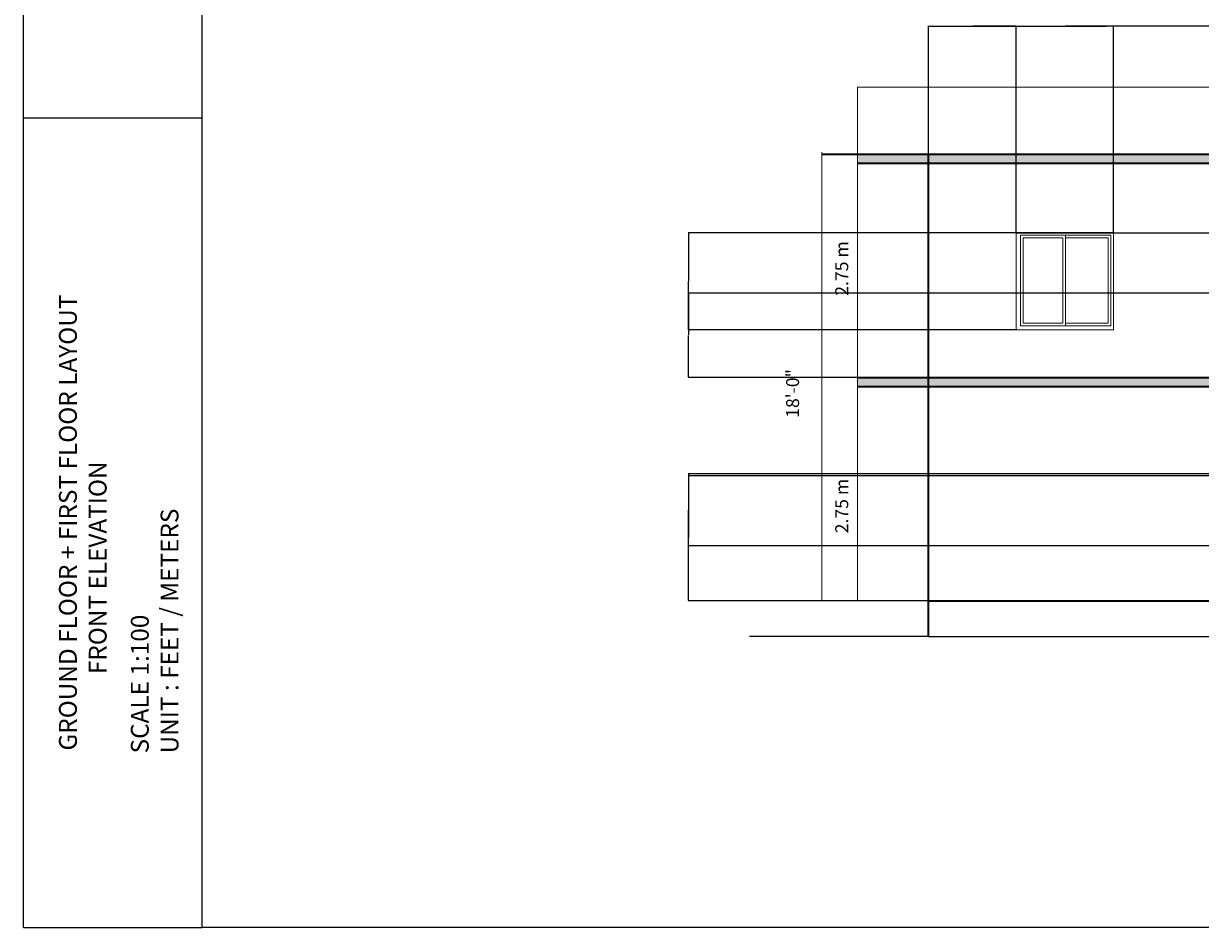
# Model space of a CAD drawing. Units: feet. Extents: x 2813 to 4435, y 1041 to 2557.
# Tile 1 of 6: x 2813 to 3605, y 1041 to 1649. Entities that reach past the tile are written whole.
import ezdxf

# ---------------------------------------------------------------- set-up
doc = ezdxf.new("R2010")
doc.units = ezdxf.units.FT
for name, color, linetype, lineweight in [('A-ANNO-DIMS', 2, 'Continuous', 18), ('A-ANNO-TTLB', 7, 'Continuous', 25), ('A-ELEV', 7, 'Continuous', 35), ('A-ELEV-GRND', 7, 'Continuous', 25), ('A-ELEV-PATT', 252, 'Continuous', 13), ('A-GLAZ', 4, 'Continuous', 18)]:
    doc.layers.add(name, color=color, linetype=linetype, lineweight=lineweight)
doc.styles.get("Standard").update_dxf_attribs({"font": 'arial.ttf'})
doc.dimstyles.get("Standard").update_dxf_attribs({"dimtxt": 0.18, "dimasz": 0.18, "dimexe": 0.18, "dimexo": 0.0625, "dimgap": 0.09, "dimtad": 0, "dimtih": 1, "dimtoh": 1, "dimdec": 4, "dimzin": 0, "dimdsep": 46, "dimtxsty": 'Standard', "dimcen": 0.09, "dimadec": 0, "dimazin": 0, "dimtfac": 1, "dimtdec": 4, "dimtofl": 0, "dimtmove": 0, "dimatfit": 3, "dimfxl": 1, "dimtolj": 1, "dimtzin": 0, "dimarcsym": 0})

# ---------------------------------------------------------------- blocks, each defined once
blk = doc.blocks.new('*U14')
for p, q in [((38.1, 38.1), (38.1, 876.3)), ((38.1, 876.3), (457.2, 876.3)), ((457.2, 38.1), (457.2, 876.3)), ((457.2, 876.3), (876.3, 876.3)), ((876.3, 876.3), (876.3, 38.1)), ((457.2, 38.1), (38.1, 38.1)), ((876.3, 38.1), (457.2, 38.1))]:
    blk.add_line(p, q)
blk.add_lwpolyline([(0, 0), (900, 0), (900, 900), (0, 900)], close=True)
for points in [[(431.8, 850.9), (431.8, 63.5), (63.5, 63.5), (63.5, 850.9), (431.8, 850.9)], [(457.2, 850.9), (850.9, 850.9), (850.9, 63.5), (457.2, 63.5)]]:
    blk.add_lwpolyline(points)
blk = doc.blocks.new('*D35')
at = {"layer": 'A-ANNO-DIMS', "color": 0, "lineweight": -2, "transparency": 16777216}
for p, q in [((3421.71, 1261.18), (3421.71, 1647.39)), ((3421.89, 1647.21), (3541.42, 1647.21)), ((3661.53, 1647.21), (3542, 1647.21)), ((3661.71, 1261.18), (3661.71, 1647.39))]:
    blk.add_line(p, q, dxfattribs=at)
at = {"layer": 'A-ANNO-DIMS', "color": 0, "transparency": 16777216}
for points in [[(3421.89, 1647.24), (3421.89, 1647.18), (3421.71, 1647.21)], [(3661.53, 1647.24), (3661.53, 1647.18), (3661.71, 1647.21)]]:
    blk.add_solid(points, dxfattribs=at)
at = {"layer": 'DEFPOINTS', "color": 0, "transparency": 16777216}
for p in [(3661.71, 1647.21), (3421.71, 1261.11), (3661.71, 1261.11)]:
    blk.add_point(p, dxfattribs=at)
at = {"layer": 'A-ANNO-DIMS', "color": 0, "transparency": 16777216, "insert": (3541.71, 1647.21), "char_height": 0.18, "attachment_point": 5}
blk.add_mtext('\\A1;240', dxfattribs=at)
blk = doc.blocks.new('*D39')
at = {"layer": 'A-ANNO-DIMS', "color": 0, "lineweight": -2, "transparency": 16777216}
for p, q in [((3421.71, 1561.18), (3421.71, 1647.39)), ((3421.89, 1647.21), (3450.85, 1647.21)), ((3480.6, 1647.21), (3451.64, 1647.21)), ((3480.78, 1508.52), (3480.78, 1647.39))]:
    blk.add_line(p, q, dxfattribs=at)
at = {"layer": 'A-ANNO-DIMS', "color": 0, "transparency": 16777216}
for points in [[(3421.89, 1647.24), (3421.89, 1647.18), (3421.71, 1647.21)], [(3480.6, 1647.24), (3480.6, 1647.18), (3480.78, 1647.21)]]:
    blk.add_solid(points, dxfattribs=at)
at = {"layer": 'DEFPOINTS', "color": 0, "transparency": 16777216}
for p in [(3480.78, 1647.21), (3421.71, 1561.11), (3480.78, 1508.46)]:
    blk.add_point(p, dxfattribs=at)
at = {"layer": 'A-ANNO-DIMS', "color": 0, "transparency": 16777216, "insert": (3451.24, 1647.21), "char_height": 0.18, "attachment_point": 5}
blk.add_mtext('\\A1;59.07', dxfattribs=at)
blk = doc.blocks.new('*D40')
at = {"layer": 'A-ANNO-DIMS', "color": 0, "lineweight": -2, "transparency": 16777216}
for p, q in [((3480.78, 1508.52), (3480.78, 1647.39)), ((3480.96, 1647.21), (3513.08, 1647.21)), ((3545.98, 1647.21), (3513.87, 1647.21)), ((3546.16, 1508.52), (3546.16, 1647.39))]:
    blk.add_line(p, q, dxfattribs=at)
at = {"layer": 'A-ANNO-DIMS', "color": 0, "transparency": 16777216}
for points in [[(3480.96, 1647.24), (3480.96, 1647.18), (3480.78, 1647.21)], [(3545.98, 1647.24), (3545.98, 1647.18), (3546.16, 1647.21)]]:
    blk.add_solid(points, dxfattribs=at)
at = {"layer": 'DEFPOINTS', "color": 0, "transparency": 16777216}
for p in [(3546.16, 1647.21), (3480.78, 1508.46), (3546.16, 1508.46)]:
    blk.add_point(p, dxfattribs=at)
at = {"layer": 'A-ANNO-DIMS', "color": 0, "transparency": 16777216, "insert": (3513.47, 1647.21), "char_height": 0.18, "attachment_point": 5}
blk.add_mtext('\\A1;65.38', dxfattribs=at)
blk = doc.blocks.new('*D43')
at = {"layer": 'A-ANNO-DIMS', "color": 0, "lineweight": -2, "transparency": 16777216}
for p, q in [((3661.64, 1345.11), (3260.3, 1345.11)), ((3260.48, 1344.93), (3260.48, 1303.3)), ((3260.48, 1261.29), (3260.48, 1302.93)), ((3661.64, 1261.11), (3260.3, 1261.11))]:
    blk.add_line(p, q, dxfattribs=at)
at = {"layer": 'A-ANNO-DIMS', "color": 0, "transparency": 16777216}
for points in [[(3260.45, 1344.93), (3260.51, 1344.93), (3260.48, 1345.11)], [(3260.45, 1261.29), (3260.51, 1261.29), (3260.48, 1261.11)]]:
    blk.add_solid(points, dxfattribs=at)
at = {"layer": 'DEFPOINTS', "color": 0, "transparency": 16777216}
for p in [(3260.48, 1345.11), (3661.71, 1345.11), (3661.71, 1261.11)]:
    blk.add_point(p, dxfattribs=at)
at = {"layer": 'A-ANNO-DIMS', "color": 0, "transparency": 16777216, "insert": (3260.48, 1303.11), "char_height": 0.18, "attachment_point": 5}
blk.add_mtext('\\A1;84', dxfattribs=at)
blk = doc.blocks.new('*D45')
at = {"layer": 'A-ANNO-DIMS', "color": 0, "lineweight": -2, "transparency": 16777216}
for p, q in [((3780.14, 1346.29), (3260.3, 1346.29)), ((3260.48, 1346.11), (3260.48, 1322.29)), ((3260.48, 1298.09), (3260.48, 1321.92)), ((3780.14, 1297.91), (3260.3, 1297.91))]:
    blk.add_line(p, q, dxfattribs=at)
at = {"layer": 'A-ANNO-DIMS', "color": 0, "transparency": 16777216}
for points in [[(3260.45, 1346.11), (3260.51, 1346.11), (3260.48, 1346.29)], [(3260.45, 1298.09), (3260.51, 1298.09), (3260.48, 1297.91)]]:
    blk.add_solid(points, dxfattribs=at)
at = {"layer": 'DEFPOINTS', "color": 0, "transparency": 16777216}
for p in [(3260.48, 1346.29), (3780.21, 1346.29), (3780.21, 1297.91)]:
    blk.add_point(p, dxfattribs=at)
at = {"layer": 'A-ANNO-DIMS', "color": 0, "transparency": 16777216, "insert": (3260.48, 1322.1), "char_height": 0.18, "attachment_point": 5}
blk.add_mtext('\\A1;48.38', dxfattribs=at)
blk = doc.blocks.new('*D46')
at = {"layer": 'A-ANNO-DIMS', "color": 0, "lineweight": -2, "transparency": 16777216}
for p, q in [((3480.72, 1508.46), (3260.3, 1508.46)), ((3260.48, 1508.28), (3260.48, 1475.95)), ((3260.48, 1443.26), (3260.48, 1475.59)), ((3480.72, 1443.08), (3260.3, 1443.08))]:
    blk.add_line(p, q, dxfattribs=at)
at = {"layer": 'A-ANNO-DIMS', "color": 0, "transparency": 16777216}
for points in [[(3260.45, 1508.28), (3260.51, 1508.28), (3260.48, 1508.46)], [(3260.45, 1443.26), (3260.51, 1443.26), (3260.48, 1443.08)]]:
    blk.add_solid(points, dxfattribs=at)
at = {"layer": 'DEFPOINTS', "color": 0, "transparency": 16777216}
for p in [(3260.48, 1508.46), (3480.78, 1508.46), (3480.78, 1443.08)]:
    blk.add_point(p, dxfattribs=at)
at = {"layer": 'A-ANNO-DIMS', "color": 0, "transparency": 16777216, "insert": (3260.48, 1475.77), "char_height": 0.18, "attachment_point": 5}
blk.add_mtext('\\A1;65.38', dxfattribs=at)
blk = doc.blocks.new('*D47')
at = {"layer": 'A-ANNO-DIMS', "color": 0, "lineweight": -2, "transparency": 16777216}
for p, q in [((3421.77, 1561.11), (4024.11, 1561.11)), ((4023.93, 1560.93), (4023.93, 1534.97)), ((4023.93, 1508.64), (4023.93, 1534.61)), ((3480.84, 1508.46), (4024.11, 1508.46))]:
    blk.add_line(p, q, dxfattribs=at)
at = {"layer": 'A-ANNO-DIMS', "color": 0, "transparency": 16777216}
for points in [[(4023.9, 1560.93), (4023.96, 1560.93), (4023.93, 1561.11)], [(4023.9, 1508.64), (4023.96, 1508.64), (4023.93, 1508.46)]]:
    blk.add_solid(points, dxfattribs=at)
at = {"layer": 'DEFPOINTS', "color": 0, "transparency": 16777216}
for p in [(3421.71, 1561.11), (3480.78, 1508.46), (4023.93, 1508.46)]:
    blk.add_point(p, dxfattribs=at)
at = {"layer": 'A-ANNO-DIMS', "color": 0, "transparency": 16777216, "insert": (4023.93, 1534.79), "char_height": 0.18, "attachment_point": 5}
blk.add_mtext('\\A1;52.65', dxfattribs=at)
blk = doc.blocks.new('*D49')
at = {"layer": 'A-ANNO-DIMS', "color": 0, "lineweight": -2, "transparency": 16777216}
for p, q in [((3732.12, 1467.89), (3260.3, 1467.89)), ((3260.48, 1467.71), (3260.48, 1439.68)), ((3260.48, 1411.29), (3260.48, 1439.32)), ((3732.12, 1411.11), (3260.3, 1411.11))]:
    blk.add_line(p, q, dxfattribs=at)
at = {"layer": 'A-ANNO-DIMS', "color": 0, "transparency": 16777216}
for points in [[(3260.45, 1467.71), (3260.51, 1467.71), (3260.48, 1467.89)], [(3260.45, 1411.29), (3260.51, 1411.29), (3260.48, 1411.11)]]:
    blk.add_solid(points, dxfattribs=at)
at = {"layer": 'DEFPOINTS', "color": 0, "transparency": 16777216}
for p in [(3260.48, 1467.89), (3732.18, 1467.89), (3732.18, 1411.11)]:
    blk.add_point(p, dxfattribs=at)
at = {"layer": 'A-ANNO-DIMS', "color": 0, "transparency": 16777216, "insert": (3260.48, 1439.5), "char_height": 0.18, "attachment_point": 5}
blk.add_mtext('\\A1;56.77', dxfattribs=at)

msp = doc.modelspace()

# ---------------------------------------------------------------- hatches: boundary and pattern name
at = {"layer": 'A-ELEV-PATT'}
h = msp.add_hatch(color=256, dxfattribs=at)
h.dxf.hatch_style = 1
h.paths.add_polyline_path([(3732.181, 1561.114), (3421.706, 1561.114), (3421.706, 1555.114), (3732.181, 1555.114)])
h.paths.add_polyline_path([(3910.706, 1561.114), (3901.706, 1561.114), (3751.395, 1561.114), (3751.395, 1555.114), (3901.706, 1555.114), (3910.706, 1555.114)])
h.paths.add_polyline_path([(3751.395, 1561.114), (3732.181, 1561.114), (3732.181, 1555.114), (3751.395, 1555.114)])
h.paths.add_polyline_path([(3421.706, 1561.114), (3374.104, 1561.114), (3374.104, 1555.114), (3421.706, 1555.114)])
h.paths.add_polyline_path([(3901.706, 1411.114), (3732.181, 1411.114), (3421.706, 1411.114), (3421.706, 1405.114), (3901.706, 1405.114)])
h.paths.add_polyline_path([(3421.706, 1411.114), (3374.104, 1411.114), (3374.104, 1405.114), (3421.706, 1405.114)])

# ---------------------------------------------------------------- linework, layer by layer
at = {"layer": 'A-ANNO-DIMS'}
for p, q in [((3374.104, 1562.484), (3374.104, 1606.165)), ((3374.104, 1606.165), (3910.706, 1606.165)), ((3350.104, 1261.114), (3350.104, 1562.484)), ((3374.104, 1261.114), (3374.104, 1562.484)), ((3421.706, 1261.114), (3350.104, 1261.114))]:
    msp.add_line(p, q, dxfattribs=at)
at = {"layer": 'A-ANNO-TTLB'}
for p, q in [((2813.466, 1041.465), (2813.466, 2556.562)), ((2933.466, 1041.465), (2933.466, 2556.562)), ((2933.466, 1585.487), (2813.466, 1585.487)), ((2813.466, 1041.465), (2933.466, 1041.465)), ((4435.474, 1041.465), (2933.466, 1041.465))]:
    msp.add_line(p, q, dxfattribs=at)
at = {"layer": 'A-ELEV'}
for p, q in [((3350.104, 1561.114), (3901.706, 1561.114)), ((3421.706, 1237.114), (3421.706, 1561.114)), ((3374.104, 1555.114), (3901.706, 1555.114)), ((3374.104, 1411.114), (3910.706, 1411.114)), ((3374.104, 1405.114), (3901.706, 1405.114)), ((3421.706, 1261.114), (3901.706, 1261.114))]:
    msp.add_line(p, q, dxfattribs=at)
at = {"layer": 'A-ELEV-GRND'}
for p, q in [((3367.017, 1237.114), (3301.526, 1237.114)), ((3421.706, 1237.114), (3367.017, 1237.114)), ((3421.706, 1237.114), (3901.706, 1237.114))]:
    msp.add_line(p, q, dxfattribs=at)

# ---------------------------------------------------------------- block references
at = {"layer": 'A-GLAZ', "xscale": 0.0726490227887824, "yscale": 0.0726490227887824, "zscale": 0.0726490227887824}
msp.add_blockref('*U14', (3480.779, 1443.078), dxfattribs=at)

# ---------------------------------------------------------------- texts
at = {"layer": 'A-ANNO-DIMS', "char_height": 8.6905, "attachment_point": 1, "rotation": 90}
for s, insert in [('2.75 m', (3359.137, 1466.059)), ('18\'-0"', (3326.1, 1384.018)), ('2.75 m', (3359.137, 1306.378))]:
    msp.add_mtext_dynamic_manual_height_columns(s, width=48.78405, gutter_width=43.452, heights=[0], dxfattribs=dict(at, insert=insert))
at = {"layer": 'A-ANNO-TTLB', "char_height": 12, "attachment_point": 1, "rotation": 90}
for s, insert in [('GROUND FLOOR + FIRST FLOOR LAYOUT\\P              FRONT ELEVATION', (2837.306, 1160.374)), ('SCALE 1:100\\PUNIT : FEET / METERS', (2885.617, 1158.445))]:
    msp.add_mtext_dynamic_manual_height_columns(s, width=375.25864, gutter_width=7.02, heights=[0], dxfattribs=dict(at, insert=insert))

# ---------------------------------------------------------------- dimensions: what is measured, and where the dimension line sits
at = {"layer": 'A-ANNO-DIMS'}
for base, p1, p2, override, picture, middle in [((3661.706, 1647.215), (3421.706, 1261.114), (3661.706, 1261.114), {"dimdec": 0, "dimlfac": 1, "dimrnd": 0, "dimzin": 0, "dimdsep": 46, "dimlunit": 2}, '*D35', (3541.706, 1647.215)), ((3480.779, 1647.215), (3421.706, 1561.114), (3480.779, 1508.462), {"dimdec": 2, "dimlfac": 1, "dimrnd": 0, "dimzin": 0, "dimdsep": 46, "dimlunit": 2}, '*D39', (3451.242, 1647.215)), ((3546.163, 1647.215), (3480.779, 1508.462), (3546.163, 1508.462), {"dimdec": 2, "dimlfac": 1, "dimrnd": 0, "dimzin": 0, "dimdsep": 46, "dimlunit": 2}, '*D40', (3513.471, 1647.215))]:
    dim = msp.add_linear_dim(base=base, p1=p1, p2=p2, dimstyle='Standard', override=override, dxfattribs=at)
    dim.commit()
    dim.dimension.update_dxf_attribs({"geometry": picture, "text_midpoint": middle})
for base, p1, p2, override, picture, middle in [((4023.932, 1508.462), (3421.706, 1561.114), (3480.779, 1508.462), {"dimdec": 2, "dimlfac": 1, "dimrnd": 0, "dimzin": 0, "dimdsep": 46, "dimlunit": 2}, '*D47', (4023.932, 1534.788)), ((3260.476, 1508.462), (3480.779, 1443.078), (3480.779, 1508.462), {"dimdec": 2, "dimlfac": 1, "dimrnd": 0, "dimzin": 0, "dimdsep": 46, "dimlunit": 2}, '*D46', (3260.476, 1475.77)), ((3260.476, 1467.886), (3732.181, 1411.114), (3732.181, 1467.886), {"dimdec": 2, "dimlfac": 1, "dimrnd": 0, "dimzin": 0, "dimdsep": 46, "dimlunit": 2}, '*D49', (3260.476, 1439.5)), ((3260.476, 1346.294), (3780.205, 1297.915), (3780.205, 1346.294), {"dimdec": 2, "dimlfac": 1, "dimrnd": 0, "dimzin": 0, "dimdsep": 46, "dimlunit": 2}, '*D45', (3260.476, 1322.104)), ((3260.476, 1345.114), (3661.706, 1261.114), (3661.706, 1345.114), {"dimdec": 0, "dimlfac": 1, "dimrnd": 0, "dimzin": 0, "dimdsep": 46, "dimlunit": 2}, '*D43', (3260.476, 1303.114))]:
    dim = msp.add_linear_dim(base=base, p1=p1, p2=p2, angle=90, dimstyle='Standard', override=override, dxfattribs=at)
    dim.commit()
    dim.dimension.update_dxf_attribs({"geometry": picture, "text_midpoint": middle})

doc.saveas('drawing.dxf')
